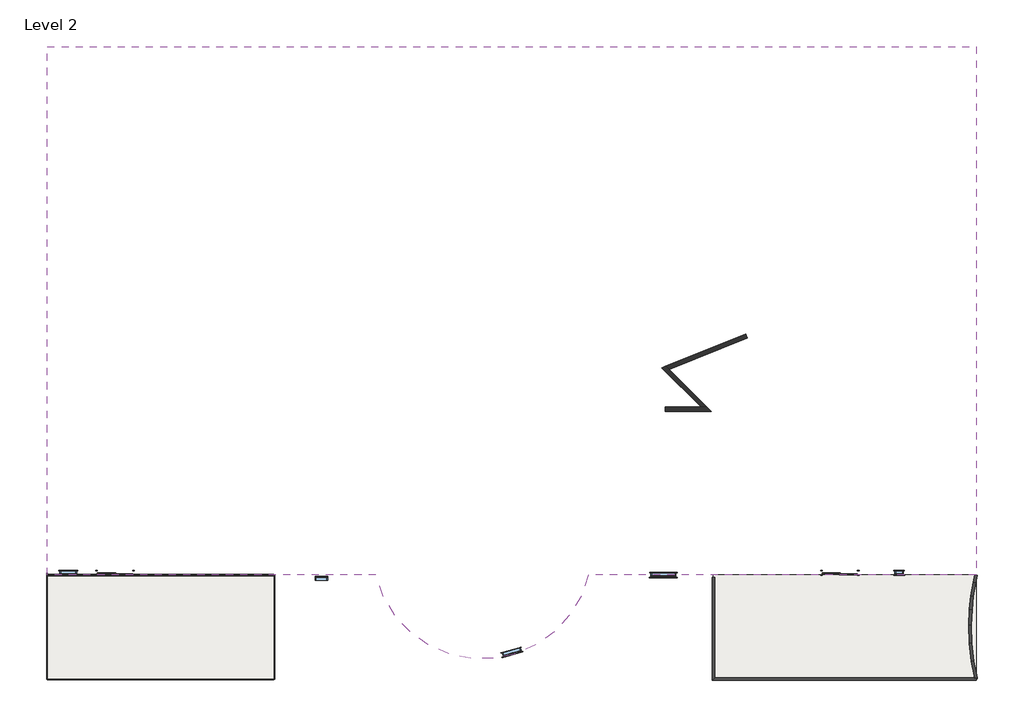
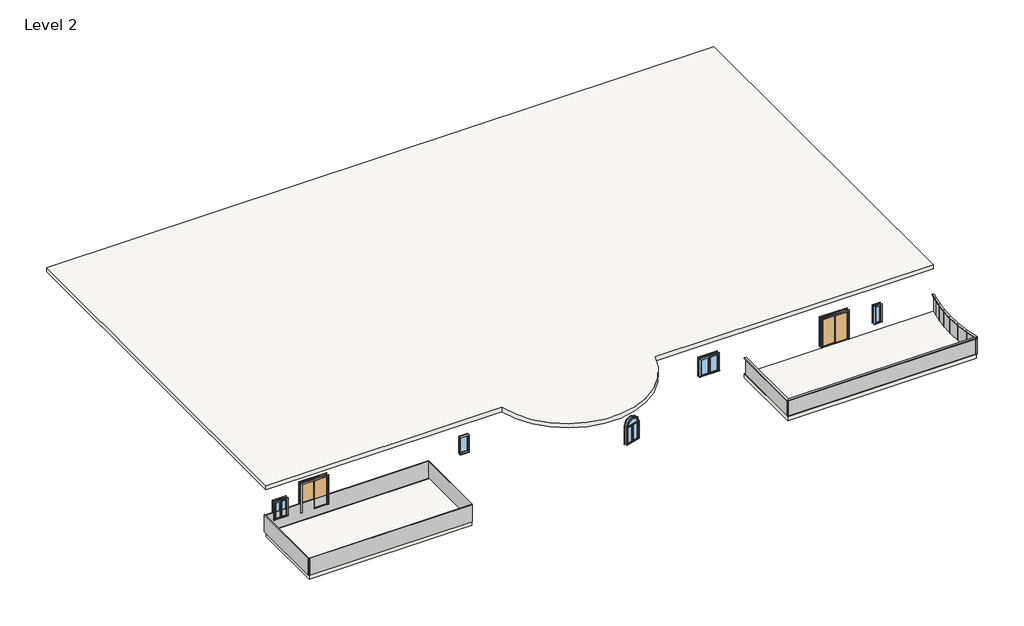
# One storey: 13 plates, 10 members, 5 windows, 3 slabs, 3 walls, 2 doors.
"""IFC4 building model written with IfcOpenShell, lengths in millimetres."""

from ifc_helpers import new_model, si_unit, point, frame, frame_2d, origin, place, context, project, spatial, polyline, circle_curve, trimmed, segment, composite_curve, outline, extrude, faceted_brep, transform, mapped, element, save
from components import door_076b30e0, member_75074519, member_1aee267e, member_b12940b7, member_3197f2db, member_0d2ca346, member_6fafe7ef, member_9a7a48cf, member_868818ab, member_d319704e, member_fc190105, system_panel_glazed_7cd9bc56, system_panel_glazed_c821ef0e, system_panel_glazed_f0dacc13, system_panel_glazed_fa5755b7, system_panel_glazed_3b0fd0dd, system_panel_glazed_b08a8559, system_panel_glazed_8842d65e, system_panel_glazed_b96adab1, system_panel_glazed_08041df1, system_panel_glazed_cbf88504, window_cf4adaea, window_a765b88f, window_bb17773d, window_0862ab64, window_80bd9af0

model = new_model("IFC4")

# Units and contexts
model_context = context("Model", 3, world=origin())
ifc_project = project(units=[si_unit("LENGTHUNIT", "METRE", prefix="MILLI")], contexts=[model_context])

# Site, building, storey
site = spatial("IfcSite", under=ifc_project)
building = spatial("IfcBuilding", under=site)
storey = spatial("IfcBuildingStorey", under=building, Name="Level 2", Elevation=3048.0)

# Doors
placement = place(None, origin())
door_shape = door_076b30e0(model_context)
element("IfcDoor", 1, ObjectType="Door-Double-Sliding : 68\" x 80\"", at=placement, inside=storey, context=model_context, shape_type="MappedRepresentation", body=[
    mapped(door_shape, transform((-16521.785279, -12227.7237084, 3592.1911771), x_axis=(-1.0, 0.0, 0.0), y_axis=(0.0, -1.0, 0.0), z_axis=(0.0, 0.0, 1.0))),
])
element("IfcDoor", 2, ObjectType="Door-Double-Sliding : 68\" x 80\"", at=placement, inside=storey, context=model_context, shape_type="MappedRepresentation", body=[
    mapped(door_shape, transform((18835.014721, -12227.7237084, 3048.0), x_axis=(-1.0, 0.0, 0.0), y_axis=(0.0, -1.0, 0.0), z_axis=(0.0, 0.0, 1.0))),
])

# Members
member_shape = member_75074519(model_context)
element("IfcMember", 3, ObjectType="Rectangular Mullion : 2.5\" x 5\" rectangular", at=placement, inside=storey, context=model_context, shape_type="MappedRepresentation", body=[
    mapped(member_shape, transform((25489.814721, -17534.921855, 3048.0), x_axis=(0.19348069679811888, -0.9811040821271281, 0.0), y_axis=(-0.9811040821271281, -0.19348069679811888, 0.0), z_axis=(0.0, 0.0, -1.0))),
])
member_2_shape = member_1aee267e(model_context)
element("IfcMember", 4, ObjectType="Rectangular Mullion : 2.5\" x 5\" rectangular", at=placement, inside=storey, context=model_context, shape_type="MappedRepresentation", body=[
    mapped(member_2_shape, transform((25295.1878978, -13483.0195767, 4267.2), x_axis=(0.0, 0.0, 1.0), y_axis=(-0.9856033837275643, 0.1690738595548575, 0.0), z_axis=(-0.1690738595548575, -0.9856033837275643, 0.0))),
])
member_3_shape = member_b12940b7(model_context)
element("IfcMember", 5, ObjectType="Rectangular Mullion : 2.5\" x 5\" rectangular", at=placement, inside=storey, context=model_context, shape_type="MappedRepresentation", body=[
    mapped(member_3_shape, transform((25318.6391414, -16666.9228111, 4267.2), x_axis=(0.0, 0.0, 1.0), y_axis=(-0.9935718556765879, -0.1132032137679038, 0.0), z_axis=(0.1132032137679038, -0.9935718556765879, 0.0))),
])
member_4_shape = member_3197f2db(model_context)
element("IfcMember", 6, ObjectType="Rectangular Mullion : 2.5\" x 5\" rectangular", at=placement, inside=storey, context=model_context, shape_type="MappedRepresentation", body=[
    mapped(member_4_shape, transform((25218.4863818, -15787.8933213, 4267.2), x_axis=(0.0, 0.0, 1.0), y_axis=(-0.9994821348031908, -0.032178598621697384, 0.0), z_axis=(0.032178598621697384, -0.9994821348031908, 0.0))),
])
member_5_shape = member_0d2ca346(model_context)
element("IfcMember", 7, ObjectType="Rectangular Mullion : 2.5\" x 5\" rectangular", at=placement, inside=storey, context=model_context, shape_type="MappedRepresentation", body=[
    mapped(member_5_shape, transform((25190.0174422, -14903.6349096, 4267.2), x_axis=(0.0, 0.0, 1.0), y_axis=(-0.9990603818624579, 0.04333997453667596, 0.0), z_axis=(-0.04333997453667596, -0.9990603818624579, 0.0))),
])
member_6_shape = member_6fafe7ef(model_context)
element("IfcMember", 8, ObjectType="Rectangular Mullion : 2.5\" x 5\" rectangular", at=placement, inside=storey, context=model_context, shape_type="MappedRepresentation", body=[
    mapped(member_6_shape, transform((25222.9611632, -14144.2259156, 4267.2), x_axis=(0.0, 0.0, 1.0), y_axis=(-0.9940867469401675, 0.10858885558801867, 0.0), z_axis=(-0.10858885558801867, -0.9940867469401675, 0.0))),
])
member_7_shape = member_9a7a48cf(model_context)
element("IfcMember", 9, ObjectType="Rectangular Mullion : 2.5\" x 5\" rectangular", at=placement, inside=storey, context=model_context, shape_type="MappedRepresentation", body=[
    mapped(member_7_shape, transform((25407.6455963, -12827.4558575, 4267.2), x_axis=(0.0, 0.0, 1.0), y_axis=(-0.9763565021870608, 0.21616655762871373, 0.0), z_axis=(-0.21616655762871373, -0.9763565021870608, 0.0))),
])
member_8_shape = member_868818ab(model_context)
element("IfcMember", 10, ObjectType="Rectangular Mullion : 2.5\" x 5\" rectangular", at=placement, inside=storey, context=model_context, shape_type="MappedRepresentation", body=[
    mapped(member_8_shape, transform((25477.5286967, -17472.6217458, 4267.2), x_axis=(0.0, 0.0, 1.0), y_axis=(-0.9811040821271279, -0.19348069679811983, 0.0), z_axis=(0.1934806967981198, -0.9811040821271277, 0.0))),
])
member_9_shape = member_d319704e(model_context)
element("IfcMember", 11, ObjectType="Rectangular Mullion : 2.5\" x 5\" rectangular", at=placement, inside=storey, context=model_context, shape_type="MappedRepresentation", body=[
    mapped(member_9_shape, transform((12667.5594464, -17534.921855, 4267.2), x_axis=(0.0, 0.0, 1.0), y_axis=(-1.0, 0.0, 0.0), z_axis=(0.0, -1.0, 0.0))),
])
member_10_shape = member_fc190105(model_context)
element("IfcMember", 12, ObjectType="Rectangular Mullion : 2.5\" x 5\" rectangular", at=placement, inside=storey, context=model_context, shape_type="MappedRepresentation", body=[
    mapped(member_10_shape, transform((25489.814721, -17534.921855, 4267.2), x_axis=(0.0, 0.0, 1.0), y_axis=(0.0, -1.0, 0.0), z_axis=(1.0, 0.0, 0.0))),
])

# Plates
system_panel_glazed_shape = system_panel_glazed_7cd9bc56(model_context)
element("IfcPlate", 13, ObjectType="System Panel : Glazed", at=placement, inside=storey, context=model_context, shape_type="MappedRepresentation", body=[
    mapped(system_panel_glazed_shape, transform((19078.6870837, -17534.921855, 3048.0), x_axis=(1.0, 0.0, 0.0), y_axis=(0.0, 1.0, 0.0), z_axis=(0.0, 0.0, 1.0))),
])
system_panel_glazed_2_shape = system_panel_glazed_c821ef0e(model_context)
element("IfcPlate", 14, ObjectType="System Panel : Glazed", at=placement, inside=storey, context=model_context, shape_type="MappedRepresentation", body=[
    mapped(system_panel_glazed_2_shape, transform((25448.7301587, -12641.889783, 3048.0), x_axis=(-0.2161665576287187, -0.9763565021870597, 0.0), y_axis=(0.9763565021870597, -0.2161665576287187, 0.0), z_axis=(0.0, 0.0, 1.0))),
])
system_panel_glazed_3_shape = system_panel_glazed_f0dacc13(model_context)
element("IfcPlate", 15, ObjectType="System Panel : Glazed", at=placement, inside=storey, context=model_context, shape_type="MappedRepresentation", body=[
    mapped(system_panel_glazed_3_shape, transform((25351.4167471, -13155.2377171, 3048.0), x_axis=(-0.1690738595548564, -0.9856033837275645, 0.0), y_axis=(0.9856033837275645, -0.1690738595548564, 0.0), z_axis=(0.0, 0.0, 1.0))),
])
element("IfcPlate", 16, ObjectType="System Panel : Glazed", at=placement, inside=storey, context=model_context, shape_type="MappedRepresentation", body=[
    mapped(system_panel_glazed_3_shape, transform((25259.0745305, -13813.6227461, 3048.0), x_axis=(-0.10858885558801937, -0.9940867469401674, 0.0), y_axis=(0.9940867469401674, -0.10858885558801937, 0.0), z_axis=(0.0, 0.0, 1.0))),
])
system_panel_glazed_4_shape = system_panel_glazed_fa5755b7(model_context)
element("IfcPlate", 17, ObjectType="System Panel : Glazed", at=placement, inside=storey, context=model_context, shape_type="MappedRepresentation", body=[
    mapped(system_panel_glazed_4_shape, transform((25206.4893027, -14523.9304126, 3048.0), x_axis=(-0.04333997453667645, -0.9990603818624579, 0.0), y_axis=(0.9990603818624579, -0.04333997453667645, 0.0), z_axis=(0.0, 0.0, 1.0))),
])
system_panel_glazed_5_shape = system_panel_glazed_3b0fd0dd(model_context)
element("IfcPlate", 18, ObjectType="System Panel : Glazed", at=placement, inside=storey, context=model_context, shape_type="MappedRepresentation", body=[
    mapped(system_panel_glazed_5_shape, transform((25204.251912, -15345.7641155, 3048.0), x_axis=(0.03217859862169707, -0.9994821348031908, 0.0), y_axis=(0.9994821348031908, 0.03217859862169707, 0.0), z_axis=(0.0, 0.0, 1.0))),
])
element("IfcPlate", 19, ObjectType="System Panel : Glazed", at=placement, inside=storey, context=model_context, shape_type="MappedRepresentation", body=[
    mapped(system_panel_glazed_5_shape, transform((25268.5627616, -16227.4080662, 3048.0), x_axis=(0.11320321376790435, -0.9935718556765878, 0.0), y_axis=(0.9935718556765878, 0.11320321376790435, 0.0), z_axis=(0.0, 0.0, 1.0))),
])
system_panel_glazed_6_shape = system_panel_glazed_b08a8559(model_context)
element("IfcPlate", 20, ObjectType="System Panel : Glazed", at=placement, inside=storey, context=model_context, shape_type="MappedRepresentation", body=[
    mapped(system_panel_glazed_6_shape, transform((25398.0839191, -17069.7722785, 3048.0), x_axis=(0.19348069679811888, -0.9811040821271281, 0.0), y_axis=(0.9811040821271281, 0.19348069679811888, 0.0), z_axis=(0.0, 0.0, 1.0))),
])
system_panel_glazed_7_shape = system_panel_glazed_8842d65e(model_context)
element("IfcPlate", 21, ObjectType="System Panel : Glazed", at=placement, inside=storey, context=model_context, shape_type="MappedRepresentation", body=[
    mapped(system_panel_glazed_7_shape, transform((12667.5594464, -15046.4227817, 3048.0), x_axis=(0.0, -1.0, 0.0), y_axis=(1.0, 0.0, 0.0), z_axis=(0.0, 0.0, 1.0))),
])
system_panel_glazed_8_shape = system_panel_glazed_b96adab1(model_context)
element("IfcPlate", 22, ObjectType="System Panel : Glazed", at=placement, inside=storey, context=model_context, shape_type="MappedRepresentation", body=[
    mapped(system_panel_glazed_8_shape, transform((-14302.7926538, -12456.3237084, 3048.0), x_axis=(1.0, 0.0, 0.0), y_axis=(0.0, 1.0, 0.0), z_axis=(0.0, 0.0, 1.0))),
])
element("IfcPlate", 23, ObjectType="System Panel : Glazed", at=placement, inside=storey, context=model_context, shape_type="MappedRepresentation", body=[
    mapped(system_panel_glazed_8_shape, transform((-14302.7926538, -17534.921855, 3048.0), x_axis=(-1.0, 0.0, 0.0), y_axis=(0.0, -1.0, 0.0), z_axis=(0.0, 0.0, 1.0))),
])
system_panel_glazed_9_shape = system_panel_glazed_08041df1(model_context)
element("IfcPlate", 24, ObjectType="System Panel : Glazed", at=placement, inside=storey, context=model_context, shape_type="MappedRepresentation", body=[
    mapped(system_panel_glazed_9_shape, transform((-8781.8000285, -14995.6227817, 3048.0), x_axis=(0.0, -1.0, 0.0), y_axis=(1.0, 0.0, 0.0), z_axis=(0.0, 0.0, 1.0))),
])
system_panel_glazed_10_shape = system_panel_glazed_cbf88504(model_context)
element("IfcPlate", 25, ObjectType="System Panel : Glazed", at=placement, inside=storey, context=model_context, shape_type="MappedRepresentation", body=[
    mapped(system_panel_glazed_10_shape, transform((-19823.785279, -14944.8227817, 3048.0), x_axis=(0.0, 1.0, 0.0), y_axis=(-1.0, 0.0, 0.0), z_axis=(0.0, 0.0, 1.0))),
])

# Slabs
element("IfcSlab", 26, ObjectType="Generic - 12\"", at=placement, inside=storey, context=model_context, shape_type="SweptSolid", body=[
    extrude(outline(composite_curve([segment(polyline([(25489.814721, 13350.0762916), (25489.814721, -12456.3237084), (6571.5594464, -12456.3237084)]), True, "CONTINUOUS"), segment(trimmed(circle_curve(frame_2d((1385.214721, -11225.6906671)), 5330.3498284), [point((6571.5594464, -12456.3237084))], [point((-3801.1300045, -12456.3237084))], False, "CARTESIAN"), True, "CONTINUOUS"), segment(polyline([(-3801.1300045, -12456.3237084), (-19823.785279, -12456.3237084), (-19823.785279, 13350.0762916), (25489.814721, 13350.0762916)]), True, "CONTINUOUS")], self_intersect=False)), frame((0.0, 0.0, 6096.0), z_axis=(0.0, 0.0, 1.0), x_axis=(1.0, 0.0, 0.0)), (0.0, 0.0, 1.0), 304.8),
])
element("IfcSlab", 27, ObjectType="Generic - 12\"", at=placement, inside=storey, context=model_context, shape_type="SweptSolid", body=[
    extrude(outline(polyline([(25489.814721, -12456.3237084), (25489.814721, -17534.921855), (12667.5594464, -17534.921855), (12667.5594464, -12456.3237084), (25489.814721, -12456.3237084)])), frame((0.0, 0.0, 2743.2), z_axis=(0.0, 0.0, 1.0), x_axis=(1.0, 0.0, 0.0)), (0.0, 0.0, 1.0), 304.8),
])
element("IfcSlab", 28, ObjectType="Generic - 12\"", at=placement, inside=storey, context=model_context, shape_type="SweptSolid", body=[
    extrude(outline(polyline([(-19823.785279, -12515.6007309), (-8781.8000285, -12515.6007309), (-8781.8000285, -17534.921855), (-19823.785279, -17534.921855), (-19823.785279, -12515.6007309)])), frame((0.0, 0.0, 2743.2), z_axis=(0.0, 0.0, 1.0), x_axis=(1.0, 0.0, 0.0)), (0.0, 0.0, 1.0), 304.8),
])

# Walls
element("IfcWall", 29, ObjectType="Generic - 8\"", at=placement, inside=storey, context=model_context, shape_type="Brep", body=[
    faceted_brep([(10331.361284, -4460.37178, 3048.0), (12557.8453819, -4460.37178, 3048.0), (12557.8453819, -4460.37178, 4267.2), (10331.361284, -4460.37178, 4267.2), (10331.361284, -4257.17178, 3048.0), (10331.361284, -4257.17178, 4267.2), (12067.2771861, -4257.17178, 4267.2), (12354.6453819, -4257.17178, 4267.2), (12354.6453819, -4257.17178, 3048.0), (12067.2771861, -4257.17178, 3048.0)], [[[0, 1, 2, 3]], [[4, 5, 6, 7, 8, 9]], [[1, 0, 4, 9, 8]], [[3, 2, 7, 6, 5]], [[0, 3, 5, 4]], [[2, 1, 8, 7]]]),
])
element("IfcWall", 30, ObjectType="Generic - 8\"", at=placement, inside=storey, context=model_context, shape_type="Brep", body=[
    faceted_brep([(12354.6453819, -4257.17178, 3048.0), (10511.7448289, -2414.271227, 3048.0), (10355.6521181, -2258.1785161, 3048.0), (10355.6521181, -2258.1785161, 4267.2), (10511.7448289, -2414.271227, 4267.2), (12354.6453819, -4257.17178, 4267.2), (12067.2771861, -4257.17178, 3048.0), (12067.2771861, -4257.17178, 4267.2), (10150.9777391, -2340.872333, 4267.2), (10150.9777391, -2340.872333, 3048.0)], [[[0, 1, 2, 3, 4, 5]], [[6, 7, 8, 9]], [[2, 1, 0, 6, 9]], [[5, 4, 3, 8, 7]], [[0, 5, 7, 6]], [[3, 2, 9, 8]]]),
])
element("IfcWall", 31, ObjectType="Generic - 8\"", at=placement, inside=storey, context=model_context, shape_type="SweptSolid", body=[
    extrude(outline(polyline([(14325.9002581, -873.2524042), (10511.7448289, -2414.271227), (10355.6521181, -2258.1785161), (14249.7801983, -684.848645), (14325.9002581, -873.2524042)])), frame((0.0, 0.0, 3048.0), z_axis=(0.0, 0.0, 1.0), x_axis=(1.0, 0.0, 0.0)), (0.0, 0.0, 1.0), 1219.2),
])

# Windows
window_shape = window_cf4adaea(model_context)
element("IfcWindow", 32, ObjectType="36\" x 48\"", at=placement, inside=storey, context=model_context, shape_type="MappedRepresentation", body=[
    mapped(window_shape, transform((2839.5240885, -16227.6735606, 3048.0), x_axis=(-0.9606648902521719, -0.2777102242208279, 0.0), y_axis=(0.2777102242208279, -0.9606648902521719, 0.0), z_axis=(0.0, 0.0, 1.0))),
])
window_2_shape = window_a765b88f(model_context)
element("IfcWindow", 33, ObjectType="Awning with Trim : 16\" x 48\"", at=placement, inside=storey, context=model_context, shape_type="MappedRepresentation", body=[
    mapped(window_2_shape, transform((21730.614721, -12354.7237084, 2600.4057153), x_axis=(-1.0, 0.0, 0.0), y_axis=(0.0, -1.0, 0.0), z_axis=(0.0, 0.0, 1.0))),
])
window_3_shape = window_bb17773d(model_context)
element("IfcWindow", 34, ObjectType="Casement Dbl with Trim : 32\" x 48\"", at=placement, inside=storey, context=model_context, shape_type="MappedRepresentation", body=[
    mapped(window_3_shape, transform((-18807.785279, -12335.6737084, 2815.6094119), x_axis=(-1.0, 0.0, 0.0), y_axis=(0.0, -1.0, 0.0), z_axis=(0.0, 0.0, 1.0))),
])
window_4_shape = window_0862ab64(model_context)
element("IfcWindow", 35, ObjectType="Casement Dbl with Trim : 48\" x 48\"", at=placement, inside=storey, context=model_context, shape_type="MappedRepresentation", body=[
    mapped(window_4_shape, transform((10229.1594464, -12437.2737084, 3048.0), x_axis=(-1.0, 0.0, 0.0), y_axis=(0.0, -1.0, 0.0), z_axis=(0.0, 0.0, 1.0))),
])
window_5_shape = window_80bd9af0(model_context)
element("IfcWindow", 36, ObjectType="Fixed : 24\" x 48\"", at=placement, inside=storey, context=model_context, shape_type="MappedRepresentation", body=[
    mapped(window_5_shape, transform((-6425.285279, -12617.2007309, 3261.0709372), x_axis=(1.0, 0.0, 0.0), y_axis=(0.0, 1.0, 0.0), z_axis=(0.0, 0.0, 1.0))),
])

save(model, "model.ifc")

# Revit data of these elements
# Type "Door-Double-Sliding : 68\" x 80\""
#   Type Mark = "10"
#   Construction Type Id = "opn-d45"
#   Assembly Code = "C1020"
#   Analytic Construction = "Wood frame, double glass door "
#   Thickness = 0' - 2"
#   Thermal Resistance (R) = 1.8150 (h·ft²·°F)/BTU
#   Heat Transfer Coefficient (U) = 0.5510 BTU/(h·ft²·°F)
#   Height = 6' - 8"
#   Rail Width = 0' - 2"
#   Stiles = 0' - 2"
#   Trim Projection Ext = 0' - 1"
#   Trim Projection Int = 0' - 1"
#   Trim Width = 0' - 3"
#   Width = 5' - 8"
#   Define Thermal Properties by = 1
#   Glazing = Glass
#   Panel Material = Wood - Birch - Solid Stained Light Low Gloss
#   Trim Material = Paint - Sienna
#   Visual Light Transmittance = 0
#   Solar Heat Gain Coefficient = 0
#   Function = (empty or 0)
#   Wall Closure = (empty or 0)
# Type "Rectangular Mullion : 2.5\" x 5\" rectangular"
#   built-in parameter 1007304 = 0.416667 (stored number, unit not read)
#   built-in parameter 1007301 = 0.104167 (stored number, unit not read)
#   built-in parameter 1007300 = 0.104167 (stored number, unit not read)
# Type "System Panel : Glazed"
#   Construction Type Id = "GSP4R"
#   Analytic Construction = "1/8 in Pilkington single glazing"
#   Visual Light Transmittance = 0.9
#   Solar Heat Gain Coefficient = 0.86
#   Heat Transfer Coefficient (U) = 1.18115 BTU/(h·ft²·°F)
# Type "Generic - 12\""
#   Assembly Code = "B1010"
#   Function = 0
#   Layers, outside or top first: 1' - 0" no material (function 1)
# Type "Generic - 8\""
#   Assembly Code = "B2010"
#   Layers, outside or top first: 0' - 8" no material (function 1)
# Type "36\" x 48\""
#   Type Mark = "38"
#   Construction Type Id = "SGL"
#   Assembly Code = "B2020100"
#   Analytic Construction = "Large single-glazed windows"
#   Visual Light Transmittance = 0.9
#   Solar Heat Gain Coefficient = 0.86
#   Heat Transfer Coefficient (U) = 0.979472 BTU/(h·ft²·°F)
#   Height = 4' - 0"
#   Default Sill Height = 3' - 0"
#   Trim Projection - Ext. = 0' - 0 1/2"
#   Trim Projection - Int. = 0' - 0 3/4"
#   Trim Width - Exterior = 0' - 3 1/2"
#   Trim Width - Interior = 0' - 3 1/2"
#   Width = 3' - 0"
#   Window Inset = 0' - 0 3/4"
#   Define Thermal Properties by = 1
#   Glass Pane Material = Glass
#   Sash Material = Sash
#   Trim Exterior Material = Trim
#   Trim Interior Material = Trim
#   Wall Closure = (empty or 0)
# Type "Awning with Trim : 16\" x 48\""
#   Type Mark = "14"
#   Construction Type Id = "GSP4R"
#   Assembly Code = "B2020100"
#   Analytic Construction = "1/8 in Pilkington single glazing"
#   Visual Light Transmittance = 0.9
#   Solar Heat Gain Coefficient = 0.78
#   Heat Transfer Coefficient (U) = 0.6496 BTU/(h·ft²·°F)
#   Height = 4' - 0"
#   Default Sill Height = 3' - 0"
#   Trim Projection - Ext. = 0' - 0 1/2"
#   Trim Projection - Int. = 0' - 0 3/4"
#   Trim Width - Exterior = 0' - 3 1/2"
#   Trim Width - Interior = 0' - 3 1/2"
#   Width = 1' - 4"
#   Window Inset = 0' - 0 3/4"
#   Define Thermal Properties by = 1
#   Glass Pane Material = Glass
#   Sash Material = Sash
#   Trim Exterior Material = Trim
#   Trim Interior Material = Trim
#   Wall Closure = (empty or 0)
# Type "Casement Dbl with Trim : 32\" x 48\""
#   Type Mark = "36"
#   Construction Type Id = "GSP4R"
#   Assembly Code = "B2020100"
#   Analytic Construction = "1/8 in Pilkington single glazing"
#   Visual Light Transmittance = 0.9
#   Solar Heat Gain Coefficient = 0.78
#   Heat Transfer Coefficient (U) = 0.6496 BTU/(h·ft²·°F)
#   Height = 4' - 0"
#   Default Sill Height = 3' - 0"
#   Trim Projection - Ext. = 0' - 0 1/2"
#   Trim Projection - Int. = 0' - 0 3/4"
#   Trim Width - Exterior = 0' - 3 1/2"
#   Trim Width - Interior = 0' - 3 1/2"
#   Width = 2' - 8"
#   Window Inset = 0' - 0 3/4"
#   Define Thermal Properties by = 1
#   Glass Pane Material = Glass
#   Sash Material = Sash
#   Trim Exterior Material = Trim
#   Trim Interior Material = Trim
#   Wall Closure = (empty or 0)
# Type "Casement Dbl with Trim : 48\" x 48\""
#   Type Mark = "34"
#   Construction Type Id = "GSP4R"
#   Assembly Code = "B2020100"
#   Analytic Construction = "1/8 in Pilkington single glazing"
#   Visual Light Transmittance = 0.9
#   Solar Heat Gain Coefficient = 0.78
#   Heat Transfer Coefficient (U) = 0.6496 BTU/(h·ft²·°F)
#   Height = 4' - 0"
#   Default Sill Height = 3' - 0"
#   Trim Projection - Ext. = 0' - 0 1/2"
#   Trim Projection - Int. = 0' - 0 3/4"
#   Trim Width - Exterior = 0' - 3 1/2"
#   Trim Width - Interior = 0' - 3 1/2"
#   Width = 4' - 0"
#   Window Inset = 0' - 0 3/4"
#   Define Thermal Properties by = 1
#   Glass Pane Material = Glass
#   Sash Material = Sash
#   Trim Exterior Material = Trim
#   Trim Interior Material = Trim
#   Wall Closure = (empty or 0)
# Type "Fixed : 24\" x 48\""
#   Type Mark = "2"
#   Construction Type Id = "GSP4R"
#   Assembly Code = "B2020100"
#   Analytic Construction = "1/8 in Pilkington single glazing"
#   Visual Light Transmittance = 0.9
#   Solar Heat Gain Coefficient = 0.78
#   Heat Transfer Coefficient (U) = 0.6496 BTU/(h·ft²·°F)
#   Height = 4' - 0"
#   Default Sill Height = 3' - 0"
#   Width = 2' - 0"
#   Window Inset = 0' - 0 3/4"
#   Define Thermal Properties by = 1
#   Glass Pane Material = Glass
#   Sash Material = Sash
#   Wall Closure = (empty or 0)
# Elements 1, 2 (IfcDoor, "Door-Double-Sliding : 68\" x 80\"")
#   Phase Created = New Construction
#   Materials on its faces: "Paint - Sienna", "Wood - Birch - Solid Stained Light Low Gloss", "Glass"
# Elements 3, 4, 5, 6, 7, 8, 9, 10, 11, 12 (IfcMember, "Rectangular Mullion : 2.5\" x 5\" rectangular")
#   Phase Created = New Construction
#   Materials on its faces: "Aluminum"
# Elements 13, 14, 15, 16, 17, 18, 19, 20, 21, 22, 23, 24, 25 (IfcPlate, "System Panel : Glazed")
#   Phase Created = New Construction
#   Materials on its faces: "Glass"
# Element 26 (IfcSlab, "Generic - 12\"")
#   Height Offset From Level = 11' - 0"
#   Phase Created = New Construction
#   Materials on its faces: "Default Floor"
# Element 27 (IfcSlab, "Generic - 12\"")
#   Height Offset From Level = 0' - 0"
#   Phase Created = New Construction
#   Materials on its faces: "Default Floor"
# Element 28 (IfcSlab, "Generic - 12\"")
#   built-in parameter 1001955 = 3.14159 (stored number, unit not read)
#   Height Offset From Level = 0' - 0"
#   Phase Created = New Construction
#   Materials on its faces: "Default Floor"
# Elements 29, 30, 31 (IfcWall, "Generic - 8\"")
#   Top Offset = 0' - 0"
#   Base Offset = 0' - 0"
#   Unconnected Height = 4' - 0"
#   wall height = 4' - 0"
#   Phase Created = New Construction
#   Base Constraint = Level 2
#   Materials on its faces: "Default Wall"
# Element 32 (IfcWindow, "36\" x 48\"")
#   Mark = "33"
#   Phase Created = New Construction
#   Materials on its faces: "Sash", "Trim", "Glass"
# Element 33 (IfcWindow, "Awning with Trim : 16\" x 48\"")
#   Mark = "67"
#   Phase Created = New Construction
#   Materials on its faces: "Sash", "Trim", "Glass"
# Element 34 (IfcWindow, "Casement Dbl with Trim : 32\" x 48\"")
#   Mark = "50"
#   Phase Created = New Construction
#   Materials on its faces: "Sash", "Trim", "Glass"
# Element 35 (IfcWindow, "Casement Dbl with Trim : 48\" x 48\"")
#   Mark = "16"
#   Phase Created = New Construction
#   Materials on its faces: "Sash", "Trim", "Glass"
# Element 36 (IfcWindow, "Fixed : 24\" x 48\"")
#   Mark = "84"
#   Phase Created = New Construction
#   Materials on its faces: "Sash", "Glass"
# Materials
#   "Glass": class "Glass", colour RGB 0 128 192, transparency 0.75, Description = "Soda Lime Glass", Cost = 0
#   "Wood - Birch - Solid Stained Light Low Gloss": class "Wood", colour RGB 210 159 95, transparency 0, Cost = 0
#   "Paint - Sienna": colour RGB 118 70 51, transparency 0, Cost = 0
#   "Sash": class "Wood", colour RGB 224 178 126, transparency 0
#   "Trim": class "Wood", colour RGB 224 178 126, transparency 0
#   "Aluminum": class "Metal", colour RGB 247 247 247, transparency 0, Description = "Aluminum 6061", Cost = 0
#   "Default Floor": colour RGB 128 128 128, transparency 0
#   "Default Wall": colour RGB 128 128 128, transparency 0
